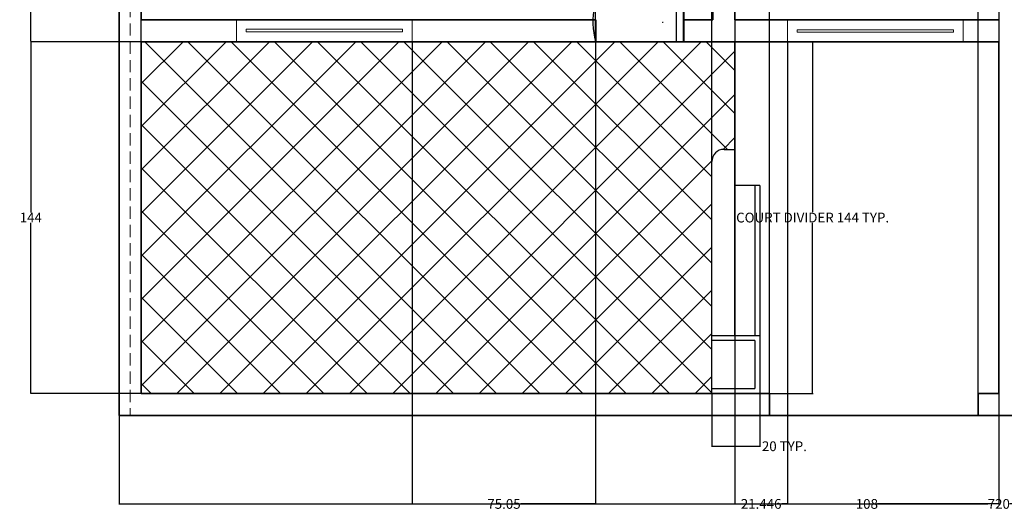
# Model space of a CAD drawing. Units: inches. Extents: x 1291 to 2095, y 532 to 1090.
# Tile 1 of 14: x 1293 to 1696, y 532 to 733. Entities that reach past the tile are written whole.
import ezdxf

# ---------------------------------------------------------------- set-up
doc = ezdxf.new("R2010")
doc.units = ezdxf.units.IN
doc.header["$MEASUREMENT"] = 0
doc.linetypes.add('HIDDEN', pattern=[0.375, 0.25, -0.125])
for name, color, linetype, lineweight in [('A-ANNO-DIMS', 2, 'Continuous', 18), ('A-DOOR', 3, 'Continuous', 25), ('A-FLOR-PATT', 252, 'Continuous', 13), ('A-GLAZ', 4, 'Continuous', 18), ('A-WALL', 7, 'Continuous', 35), ('A-WALL-HIDN', 8, 'HIDDEN', 13), ('A-WALL-SITE', 7, 'Continuous', 25)]:
    doc.layers.add(name, color=color, linetype=linetype, lineweight=lineweight)
doc.styles.get("Standard").update_dxf_attribs({"font": 'arial.ttf'})
doc.dimstyles.get("Standard").update_dxf_attribs({"dimtxt": 4, "dimasz": 0.18, "dimexe": 0.18, "dimexo": 0.0625, "dimgap": 0.09, "dimtad": 0, "dimtih": 1, "dimtoh": 1, "dimdec": 0, "dimrnd": 6, "dimzin": 0, "dimdsep": 46, "dimlunit": 3, "dimtxsty": 'Standard', "dimcen": 0.09, "dimadec": 0, "dimazin": 0, "dimtfac": 1, "dimtdec": 0, "dimtofl": 0, "dimtmove": 0, "dimatfit": 3, "dimfxl": 1, "dimtolj": 1, "dimtzin": 0, "dimarcsym": 0})

# ---------------------------------------------------------------- blocks, each defined once
blk = doc.blocks.new('WIN-72IN')
for points in [[(0, 0), (0, 9), (72, 9), (72, 0)], [(4, 4), (4, 5), (68, 5), (68, 4)]]:
    blk.add_lwpolyline(points, close=True)
blk = doc.blocks.new('FRONT-COURT-DIVIDER')
for p, q in [((9.46, 23.64), (9.46, 144)), ((5, 99.92), (9.46, 99.92)), ((0, 0), (0, 94.92)), ((19.66, 85.14), (9.46, 85.14)), ((17.66, 85.14), (17.66, 23.64)), ((19.66, 85.14), (19.66, 0)), ((19.66, 23.64), (0, 23.64)), ((17.66, 21.64), (0, 21.64)), ((17.66, 21.64), (17.66, 2)), ((0, 2), (17.66, 2))]:
    blk.add_line(p, q)
blk.add_arc((5, 94.92), 5, 90, 180)
blk = doc.blocks.new('*D26')
at = {"layer": 'A-ANNO-DIMS', "color": 0, "lineweight": -2, "transparency": 16777216}
for p, q in [((1596.33, 723.78), (1618.05, 723.78)), ((1617.87, 723.6), (1617.87, 653.94)), ((1617.87, 579.96), (1617.87, 649.62)), ((1596.33, 579.78), (1618.05, 579.78))]:
    blk.add_line(p, q, dxfattribs=at)
at = {"layer": 'A-ANNO-DIMS', "color": 0, "transparency": 16777216}
for points in [[(1617.84, 723.6), (1617.9, 723.6), (1617.87, 723.78)], [(1617.84, 579.96), (1617.9, 579.96), (1617.87, 579.78)]]:
    blk.add_solid(points, dxfattribs=at)
at = {"layer": 'Defpoints', "color": 0, "transparency": 16777216}
for p in [(1596.27, 723.78), (1617.87, 723.78), (1596.27, 579.78)]:
    blk.add_point(p, dxfattribs=at)
at = {"layer": 'A-ANNO-DIMS', "color": 0, "transparency": 16777216, "insert": (1617.87, 651.78), "char_height": 4, "attachment_point": 5}
blk.add_mtext('\\A1;COURT DIVIDER 144 TYP.', dxfattribs=at)
blk = doc.blocks.new('*D27')
at = {"layer": 'A-ANNO-DIMS', "color": 0, "lineweight": -2, "transparency": 16777216}
for p, q in [((1576.61, 579.72), (1576.61, 558)), ((1596.27, 579.72), (1596.27, 558)), ((1576.79, 558.18), (1596.09, 558.18)), ((1596.27, 558.18), (1596.45, 558.18))]:
    blk.add_line(p, q, dxfattribs=at)
at = {"layer": 'A-ANNO-DIMS', "color": 0, "transparency": 16777216}
for points in [[(1576.79, 558.21), (1576.79, 558.15), (1576.61, 558.18)], [(1596.09, 558.21), (1596.09, 558.15), (1596.27, 558.18)]]:
    blk.add_solid(points, dxfattribs=at)
at = {"layer": 'Defpoints', "color": 0, "transparency": 16777216}
for p in [(1576.61, 579.78), (1596.27, 579.78), (1596.27, 558.18)]:
    blk.add_point(p, dxfattribs=at)
at = {"layer": 'A-ANNO-DIMS', "color": 0, "transparency": 16777216, "insert": (1606.31, 558.18), "char_height": 4, "attachment_point": 5}
blk.add_mtext('\\A1;20 TYP.', dxfattribs=at)
blk = doc.blocks.new('*D32')
at = {"layer": 'A-ANNO-DIMS', "color": 0, "lineweight": -2, "transparency": 16777216}
for p, q in [((1334.07, 570.72), (1334.07, 534.4)), ((2054.07, 570.72), (2054.07, 534.4)), ((1334.25, 534.58), (1689.59, 534.58)), ((2053.89, 534.58), (1698.56, 534.58))]:
    blk.add_line(p, q, dxfattribs=at)
at = {"layer": 'A-ANNO-DIMS', "color": 0, "transparency": 16777216}
for points in [[(1334.25, 534.61), (1334.25, 534.55), (1334.07, 534.58)], [(2053.89, 534.61), (2053.89, 534.55), (2054.07, 534.58)]]:
    blk.add_solid(points, dxfattribs=at)
at = {"layer": 'Defpoints', "color": 0, "transparency": 16777216}
for p in [(1334.07, 570.78), (2054.07, 570.78), (2054.07, 534.58)]:
    blk.add_point(p, dxfattribs=at)
at = {"layer": 'A-ANNO-DIMS', "color": 0, "transparency": 16777216, "insert": (1694.07, 534.58), "char_height": 4, "attachment_point": 5}
blk.add_mtext('\\A1;720', dxfattribs=at)
blk = doc.blocks.new('*D34')
at = {"layer": 'A-ANNO-DIMS', "color": 0, "lineweight": -2, "transparency": 16777216}
for p, q in [((1343.01, 723.78), (1297.69, 723.78)), ((1297.87, 723.6), (1297.87, 653.88)), ((1297.87, 579.96), (1297.87, 649.68)), ((1343.01, 579.78), (1297.69, 579.78))]:
    blk.add_line(p, q, dxfattribs=at)
at = {"layer": 'A-ANNO-DIMS', "color": 0, "transparency": 16777216}
for points in [[(1297.84, 723.6), (1297.9, 723.6), (1297.87, 723.78)], [(1297.84, 579.96), (1297.9, 579.96), (1297.87, 579.78)]]:
    blk.add_solid(points, dxfattribs=at)
at = {"layer": 'Defpoints', "color": 0, "transparency": 16777216}
for p in [(1297.87, 723.78), (1343.07, 723.78), (1343.07, 579.78)]:
    blk.add_point(p, dxfattribs=at)
at = {"layer": 'A-ANNO-DIMS', "color": 0, "transparency": 16777216, "insert": (1297.87, 651.78), "char_height": 4, "attachment_point": 5}
blk.add_mtext('\\A1;144', dxfattribs=at)
blk = doc.blocks.new('*D35')
at = {"layer": 'A-ANNO-DIMS', "color": 0, "lineweight": -2, "transparency": 16777216}
for p, q in [((1343.01, 945.78), (1297.69, 945.78)), ((1297.87, 945.6), (1297.87, 836.88)), ((1297.87, 723.96), (1297.87, 832.68)), ((1343.01, 723.78), (1297.69, 723.78))]:
    blk.add_line(p, q, dxfattribs=at)
at = {"layer": 'A-ANNO-DIMS', "color": 0, "transparency": 16777216}
for points in [[(1297.84, 945.6), (1297.9, 945.6), (1297.87, 945.78)], [(1297.84, 723.96), (1297.9, 723.96), (1297.87, 723.78)]]:
    blk.add_solid(points, dxfattribs=at)
at = {"layer": 'Defpoints', "color": 0, "transparency": 16777216}
for p in [(1297.87, 945.78), (1343.07, 945.78), (1343.07, 723.78)]:
    blk.add_point(p, dxfattribs=at)
at = {"layer": 'A-ANNO-DIMS', "color": 0, "transparency": 16777216, "insert": (1297.87, 834.78), "char_height": 4, "attachment_point": 5}
blk.add_mtext('\\A1;222', dxfattribs=at)
blk = doc.blocks.new('*D44')
at = {"layer": 'A-ANNO-DIMS', "color": 0, "lineweight": -2, "transparency": 16777216}
for p, q in [((1343.07, 579.84), (1343.07, 1087.16)), ((1343.25, 1086.98), (1451.42, 1086.98)), ((1576.43, 1086.98), (1468.26, 1086.98)), ((1576.61, 579.84), (1576.61, 1087.16))]:
    blk.add_line(p, q, dxfattribs=at)
at = {"layer": 'A-ANNO-DIMS', "color": 0, "transparency": 16777216}
for points in [[(1343.25, 1087.01), (1343.25, 1086.95), (1343.07, 1086.98)], [(1576.43, 1087.01), (1576.43, 1086.95), (1576.61, 1086.98)]]:
    blk.add_solid(points, dxfattribs=at)
at = {"layer": 'Defpoints', "color": 0, "transparency": 16777216}
for p in [(1576.61, 1086.98), (1343.07, 579.78), (1576.61, 579.78)]:
    blk.add_point(p, dxfattribs=at)
at = {"layer": 'A-ANNO-DIMS', "color": 0, "transparency": 16777216, "insert": (1459.84, 1086.98), "char_height": 4, "attachment_point": 5}
blk.add_mtext('\\A1;233.54', dxfattribs=at)
blk = doc.blocks.new('*D46')
at = {"layer": 'A-ANNO-DIMS', "color": 0, "lineweight": -2, "transparency": 16777216}
for p, q in [((1600.27, 579.84), (1600.27, 1087.16)), ((1600.45, 1086.98), (1636.47, 1086.98)), ((1685.4, 1086.98), (1649.38, 1086.98)), ((1685.58, 579.84), (1685.58, 1087.16))]:
    blk.add_line(p, q, dxfattribs=at)
at = {"layer": 'A-ANNO-DIMS', "color": 0, "transparency": 16777216}
for points in [[(1600.45, 1087.01), (1600.45, 1086.95), (1600.27, 1086.98)], [(1685.4, 1087.01), (1685.4, 1086.95), (1685.58, 1086.98)]]:
    blk.add_solid(points, dxfattribs=at)
at = {"layer": 'Defpoints', "color": 0, "transparency": 16777216}
for p in [(1685.58, 1086.98), (1600.27, 579.78), (1685.58, 579.78)]:
    blk.add_point(p, dxfattribs=at)
at = {"layer": 'A-ANNO-DIMS', "color": 0, "transparency": 16777216, "insert": (1642.93, 1086.98), "char_height": 4, "attachment_point": 5}
blk.add_mtext('\\A1;85.31', dxfattribs=at)
blk = doc.blocks.new('*D49')
at = {"layer": 'A-ANNO-DIMS', "color": 0, "lineweight": -2, "transparency": 16777216}
for p, q in [((1694.07, 852.72), (1694.07, 534.4)), ((1586.07, 816.72), (1586.07, 534.4)), ((1586.25, 534.58), (1635.75, 534.58)), ((1693.89, 534.58), (1644.4, 534.58))]:
    blk.add_line(p, q, dxfattribs=at)
at = {"layer": 'A-ANNO-DIMS', "color": 0, "transparency": 16777216}
for points in [[(1586.25, 534.61), (1586.25, 534.55), (1586.07, 534.58)], [(1693.89, 534.61), (1693.89, 534.55), (1694.07, 534.58)]]:
    blk.add_solid(points, dxfattribs=at)
at = {"layer": 'Defpoints', "color": 0, "transparency": 16777216}
for p in [(1694.07, 852.78), (1586.07, 816.78), (1694.07, 534.58)]:
    blk.add_point(p, dxfattribs=at)
at = {"layer": 'A-ANNO-DIMS', "color": 0, "transparency": 16777216, "insert": (1640.07, 534.58), "char_height": 4, "attachment_point": 5}
blk.add_mtext('\\A1;108', dxfattribs=at)
blk = doc.blocks.new('*D62')
at = {"layer": 'A-ANNO-DIMS', "color": 0, "lineweight": -2, "transparency": 16777216}
for p, q in [((1454.02, 723.78), (1454.02, 534.4)), ((1529.07, 723.72), (1529.07, 534.4)), ((1454.2, 534.58), (1484.71, 534.58)), ((1528.89, 534.58), (1498.39, 534.58))]:
    blk.add_line(p, q, dxfattribs=at)
at = {"layer": 'A-ANNO-DIMS', "color": 0, "transparency": 16777216}
for points in [[(1454.2, 534.61), (1454.2, 534.55), (1454.02, 534.58)], [(1528.89, 534.61), (1528.89, 534.55), (1529.07, 534.58)]]:
    blk.add_solid(points, dxfattribs=at)
at = {"layer": 'Defpoints', "color": 0, "transparency": 16777216}
for p in [(1454.02, 723.85), (1529.07, 723.78), (1529.07, 534.58)]:
    blk.add_point(p, dxfattribs=at)
at = {"layer": 'A-ANNO-DIMS', "color": 0, "transparency": 16777216, "insert": (1491.55, 534.58), "char_height": 4, "attachment_point": 5}
blk.add_mtext('\\A1;75.05', dxfattribs=at)
blk = doc.blocks.new('*D63')
at = {"layer": 'A-ANNO-DIMS', "color": 0, "lineweight": -2, "transparency": 16777216}
for p, q in [((1529.07, 723.84), (1529.07, 1087.16)), ((1529.25, 1086.98), (1544.12, 1086.98)), ((1564.89, 1086.98), (1550.03, 1086.98)), ((1565.07, 723.84), (1565.07, 1087.16))]:
    blk.add_line(p, q, dxfattribs=at)
at = {"layer": 'A-ANNO-DIMS', "color": 0, "transparency": 16777216}
for points in [[(1529.25, 1087.01), (1529.25, 1086.95), (1529.07, 1086.98)], [(1564.89, 1087.01), (1564.89, 1086.95), (1565.07, 1086.98)]]:
    blk.add_solid(points, dxfattribs=at)
at = {"layer": 'Defpoints', "color": 0, "transparency": 16777216}
for p in [(1565.07, 1086.98), (1529.07, 723.78), (1565.07, 723.78)]:
    blk.add_point(p, dxfattribs=at)
at = {"layer": 'A-ANNO-DIMS', "color": 0, "transparency": 16777216, "insert": (1547.07, 1086.98), "char_height": 4, "attachment_point": 5}
blk.add_mtext('\\A1;36', dxfattribs=at)
blk = doc.blocks.new('*D64')
at = {"layer": 'A-ANNO-DIMS', "color": 0, "lineweight": -2, "transparency": 16777216}
for p, q in [((1586.07, 723.72), (1586.07, 534.4)), ((1607.52, 723.57), (1607.52, 534.4)), ((1586.25, 534.58), (1588.37, 534.58)), ((1607.34, 534.58), (1605.22, 534.58))]:
    blk.add_line(p, q, dxfattribs=at)
at = {"layer": 'A-ANNO-DIMS', "color": 0, "transparency": 16777216}
for points in [[(1586.25, 534.61), (1586.25, 534.55), (1586.07, 534.58)], [(1607.34, 534.61), (1607.34, 534.55), (1607.52, 534.58)]]:
    blk.add_solid(points, dxfattribs=at)
at = {"layer": 'Defpoints', "color": 0, "transparency": 16777216}
for p in [(1586.07, 723.78), (1607.52, 723.63), (1607.52, 534.58)]:
    blk.add_point(p, dxfattribs=at)
at = {"layer": 'A-ANNO-DIMS', "color": 0, "transparency": 16777216, "insert": (1596.8, 534.58), "char_height": 4, "attachment_point": 5}
blk.add_mtext('\\A1;21.446', dxfattribs=at)
blk = doc.blocks.new('*D89')
at = {"layer": 'A-ANNO-DIMS', "color": 0, "lineweight": -2, "transparency": 16777216}
for p, q in [((1522.71, 762.72), (1522.89, 762.72)), ((1522.89, 762.72), (1535.38, 751.22)), ((1556.46, 731.72), (1556.64, 731.72)), ((1556.55, 731.63), (1556.55, 731.81))]:
    blk.add_line(p, q, dxfattribs=at)
at = {"layer": 'A-ANNO-DIMS', "color": 0, "transparency": 16777216}
blk.add_solid([(1535.4, 751.24), (1535.36, 751.2), (1535.51, 751.1)], dxfattribs=at)
at = {"layer": 'Defpoints', "color": 0, "transparency": 16777216}
for p in [(1535.51, 751.1), (1556.55, 731.72)]:
    blk.add_point(p, dxfattribs=at)
at = {"layer": 'A-ANNO-DIMS', "color": 0, "transparency": 16777216, "insert": (1515.52, 762.72), "char_height": 4, "attachment_point": 5}
blk.add_mtext('\\A1;R28.6', dxfattribs=at)

msp = doc.modelspace()

# ---------------------------------------------------------------- hatches: boundary and pattern name
at = {"layer": 'A-FLOR-PATT'}
h = msp.add_hatch(dxfattribs=at)
h.set_pattern_fill('ANSI37', color=256, scale=100)
h.paths.add_polyline_path([(1576.6107, 674.6964, -0.41421356), (1581.6107, 679.6964), (1586.0735, 679.6964), (1586.0735, 723.7804), (1565.2125, 723.7804), (1565.2125, 723.7536), (1562.2125, 723.7536), (1529.0735, 723.7804), (1343.0735, 723.7804), (1343.0735, 579.7804), (1576.6107, 579.7804)])

# ---------------------------------------------------------------- linework, layer by layer
at = {"layer": 'A-DOOR'}
msp.add_lwpolyline([(1562.2125, 759.7536), (1565.2125, 759.7536), (1565.2125, 723.7536), (1562.2125, 723.7536)], close=True, dxfattribs=at)
msp.add_arc((1556.5498, 731.7195), 28.6002, 78.580328, 196.116311, dxfattribs=at)
at = {"layer": 'A-WALL'}
for p, q in [((1334.0735, 1050.7804), (1334.0735, 570.7804)), ((1343.0735, 936.7804), (1343.0735, 732.7804)), ((1577.0735, 732.7804), (1577.0735, 816.7804)), ((1586.0735, 732.7804), (1586.0735, 816.7804)), ((1343.0735, 732.7804), (1529.0735, 732.7804)), ((1529.0735, 723.7804), (1529.0735, 732.7804)), ((1565.0735, 723.7804), (1565.0735, 732.7804)), ((1565.0735, 732.7804), (1577.0735, 732.7804)), ((1586.0735, 732.7804), (1694.0735, 732.7804)), ((1343.0735, 723.7804), (1529.0735, 723.7804)), ((1343.0735, 723.7804), (1343.0735, 579.7804)), ((1529.0735, 723.7804), (1694.0735, 723.7804)), ((1694.0735, 579.7804), (1694.0735, 723.7804)), ((1343.0735, 579.7804), (1600.2697, 579.7804)), ((1600.2697, 579.7804), (1600.2697, 570.7804)), ((1685.5842, 579.7804), (1694.0735, 579.7804)), ((1685.5842, 570.7804), (1685.5842, 579.7804)), ((1334.0735, 570.7804), (1685.5842, 570.7804)), ((1685.5842, 570.7804), (1710.3593, 570.7804))]:
    msp.add_line(p, q, dxfattribs=at)
at = {"layer": 'A-WALL-HIDN', "ltscale": 20}
msp.add_line((1338.5735, 1046.2804), (1338.5735, 570.7804), dxfattribs=at)

# ---------------------------------------------------------------- block references
at = {"layer": 'A-GLAZ'}
for p in [(1382.0238, 723.8457), (1607.5196, 723.6289)]:
    msp.add_blockref('WIN-72IN', p, dxfattribs=at)
at = {"layer": 'A-WALL-SITE'}
msp.add_blockref('FRONT-COURT-DIVIDER', (1576.611, 579.78), dxfattribs=at)

# ---------------------------------------------------------------- dimensions: what is measured, and where the dimension line sits
at = {"layer": 'A-ANNO-DIMS'}
for base, p1, p2, override, picture, middle in [((1576.6107, 1086.9804), (1343.0735, 579.7804), (1576.6107, 579.7804), {"dimdec": 2, "dimlfac": 1, "dimrnd": 0, "dimzin": 0, "dimdsep": 46, "dimlunit": 2}, '*D44', (1459.8421, 1086.9804)), ((1565.0735, 1086.9804), (1529.0735, 723.7804), (1565.0735, 723.7804), {"dimdec": 0, "dimlfac": 1, "dimrnd": 0, "dimzin": 0, "dimdsep": 46, "dimlunit": 2}, '*D63', (1547.0735, 1086.9804)), ((1685.5842, 1086.9804), (1600.2697, 579.7804), (1685.5842, 579.7804), {"dimdec": 2, "dimlfac": 1, "dimrnd": 0, "dimzin": 0, "dimdsep": 46, "dimlunit": 2}, '*D46', (1642.927, 1086.9804)), ((1694.0735, 534.5804), (1586.0735, 816.7804), (1694.0735, 852.7804), {"dimdec": 0, "dimlfac": 1, "dimrnd": 0, "dimzin": 0, "dimdsep": 46, "dimlunit": 2}, '*D49', (1640.0735, 534.5804)), ((1529.0735, 534.5804), (1454.0234, 723.8453), (1529.0735, 723.7804), {"dimdec": 2, "dimlfac": 1, "dimrnd": 0, "dimzin": 0, "dimdsep": 46, "dimlunit": 2}, '*D62', (1491.5485, 534.5804)), ((1607.5192, 534.5804), (1586.0735, 723.7804), (1607.5192, 723.6285), {"dimdec": 3, "dimlfac": 1, "dimrnd": 0, "dimzin": 0, "dimdsep": 46, "dimlunit": 2}, '*D64', (1596.7964, 534.5804)), ((2054.0735, 534.5804), (1334.0735, 570.7804), (2054.0735, 570.7804), {"dimdec": 0, "dimlfac": 1, "dimrnd": 0, "dimzin": 0, "dimdsep": 46, "dimlunit": 2}, '*D32', (1694.0735, 534.5804))]:
    dim = msp.add_linear_dim(base=base, p1=p1, p2=p2, dimstyle='Standard', override=override, dxfattribs=at)
    dim.commit()
    dim.dimension.update_dxf_attribs({"geometry": picture, "text_midpoint": middle})
for base, p1, p2, picture, middle in [((1297.8735, 945.7804), (1343.0735, 723.7804), (1343.0735, 945.7804), '*D35', (1297.8735, 834.7804)), ((1297.8735, 723.7804), (1343.0735, 579.7804), (1343.0735, 723.7804), '*D34', (1297.8735, 651.7804))]:
    dim = msp.add_linear_dim(base=base, p1=p1, p2=p2, angle=90, dimstyle='Standard', override={"dimdec": 0, "dimlfac": 1, "dimrnd": 0, "dimzin": 0, "dimdsep": 46, "dimlunit": 2}, dxfattribs=at)
    dim.commit()
    dim.dimension.update_dxf_attribs({"geometry": picture, "text_midpoint": middle})
dim = msp.add_radius_dim(center=(1556.5498, 731.7195), mpoint=(1535.5147, 751.0973), dimstyle='Standard', override={"dimdec": 1, "dimlfac": 1, "dimrnd": 0, "dimzin": 0, "dimdsep": 46, "dimlunit": 2}, dxfattribs=at)
dim.commit()
dim.dimension.update_dxf_attribs({"geometry": '*D89', "text_midpoint": (1515.5159, 762.724), "dimtype": 164})
dim = msp.add_linear_dim(base=(1617.8697, 723.7804), p1=(1596.2697, 579.7804), p2=(1596.2697, 723.7804), angle=90, text='COURT DIVIDER <> TYP.', dimstyle='Standard', override={"dimdec": 0, "dimlfac": 1, "dimrnd": 0, "dimzin": 0, "dimdsep": 46, "dimlunit": 2}, dxfattribs=at)
dim.commit()
dim.dimension.update_dxf_attribs({"geometry": '*D26', "text_midpoint": (1617.8697, 651.7804)})
dim = msp.add_linear_dim(base=(1596.2697, 558.1804), p1=(1576.6107, 579.7804), p2=(1596.2697, 579.7804), text='<> TYP.', dimstyle='Standard', override={"dimdec": 0, "dimlfac": 1, "dimrnd": 0, "dimzin": 0, "dimdsep": 46, "dimlunit": 2}, dxfattribs=at)
dim.commit()
dim.dimension.update_dxf_attribs({"geometry": '*D27', "text_midpoint": (1606.3092, 558.1804)})

doc.saveas('drawing.dxf')
